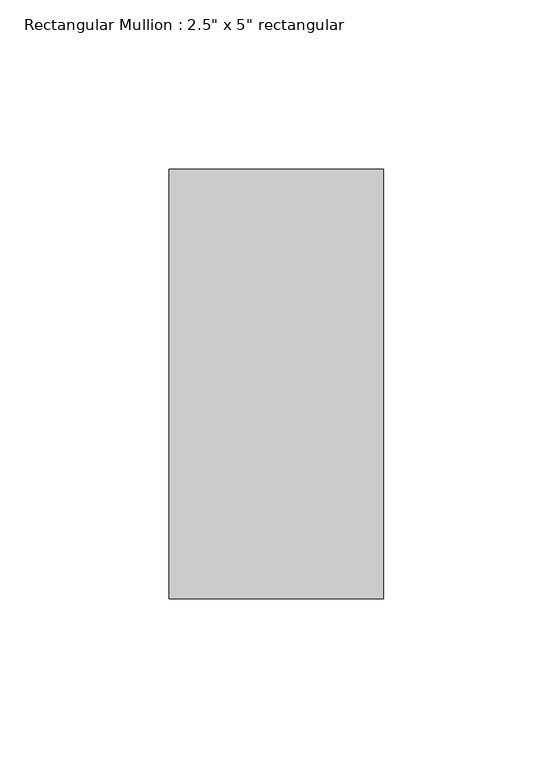
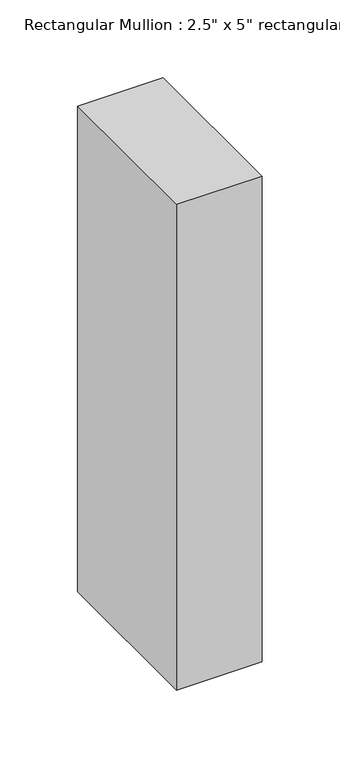
"""IFC4 building model written with IfcOpenShell, lengths in millimetres: member geometry."""

from ifc_helpers import new_model, si_unit, frame, origin, place, context, project, spatial, polyline, outline, extrude, source, transform, mapped, element, save


def member_dfe75557(model_context):
    return source(origin(), model_context, "Body", "SweptSolid", [
        extrude(outline(polyline([(0.0, 63.5), (0.0, -63.5), (-63.5, -63.5), (-63.5, 63.5), (0.0, 63.5)])), frame((0.0, 0.0, -381.0), z_axis=(0.0, 0.0, 1.0), x_axis=(1.0, 0.0, 0.0)), (0.0, 0.0, 1.0), 381.0),
    ])


if __name__ == "__main__":
    model = new_model("IFC4")
    model_context = context("Model", 3, world=origin())
    ifc_project = project(units=[si_unit("LENGTHUNIT", "METRE", prefix="MILLI")], contexts=[model_context])
    site = spatial("IfcSite", under=ifc_project)
    building = spatial("IfcBuilding", under=site)
    placement = place(None, origin())
    member_shape = member_dfe75557(model_context)
    element("IfcMember", 1, ObjectType="Rectangular Mullion : 2.5\" x 5\" rectangular", at=placement, inside=building, context=model_context, shape_type="MappedRepresentation", body=[
        mapped(member_shape, transform((0.0, 0.0, 0.0), x_axis=(1.0, 0.0, 0.0), y_axis=(0.0, 1.0, 0.0), z_axis=(0.0, 0.0, 1.0))),
    ])
    save(model, "model.ifc")

# Revit data of these elements
# Type "Rectangular Mullion : 2.5\" x 5\" rectangular"
#   built-in parameter 1007304 = 0.416667 (stored number, unit not read)
#   built-in parameter 1007301 = 0.104167 (stored number, unit not read)
#   built-in parameter 1007300 = 0.104167 (stored number, unit not read)
